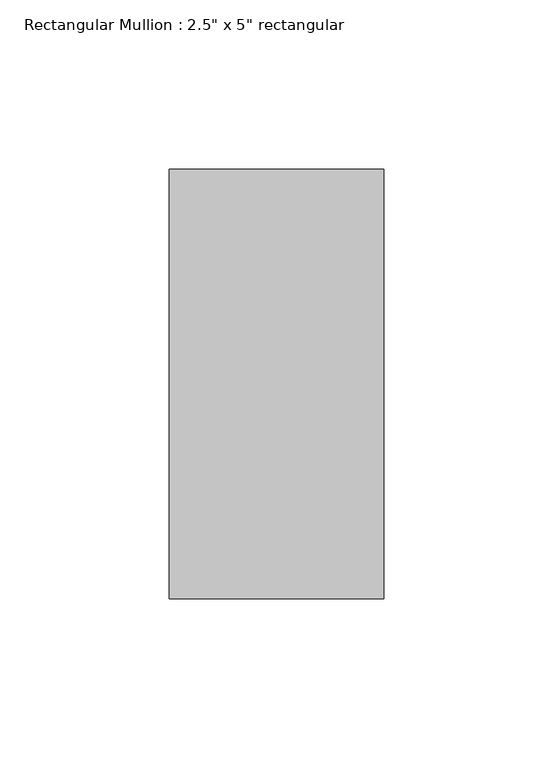
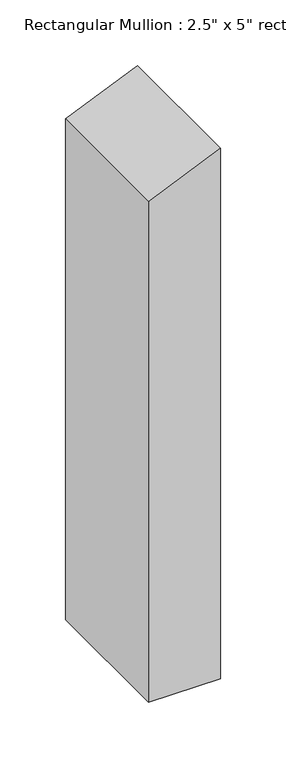
"""IFC4 building model written with IfcOpenShell, lengths in millimetres: member geometry."""

from ifc_helpers import new_model, si_unit, frame, origin, place, context, project, spatial, polyline, outline, extrude, source, transform, mapped, element, save


def member_3f5ee701(model_context):
    return source(origin(), model_context, "Body", "SweptSolid", [
        extrude(outline(polyline([(0.0, 0.0), (-27.6105858, -63.5), (-494.323108, -63.5), (-494.323108, 0.0), (0.0, 0.0)])), frame((0.0, -63.5, 0.0), z_axis=(0.0, 1.0, 0.0), x_axis=(0.0, 0.0, 1.0)), (0.0, 0.0, 1.0), 127.0),
    ])


if __name__ == "__main__":
    model = new_model("IFC4")
    model_context = context("Model", 3, world=origin())
    ifc_project = project(units=[si_unit("LENGTHUNIT", "METRE", prefix="MILLI")], contexts=[model_context])
    site = spatial("IfcSite", under=ifc_project)
    building = spatial("IfcBuilding", under=site)
    placement = place(None, origin())
    member_shape = member_3f5ee701(model_context)
    element("IfcMember", 1, ObjectType="Rectangular Mullion : 2.5\" x 5\" rectangular", at=placement, inside=building, context=model_context, shape_type="MappedRepresentation", body=[
        mapped(member_shape, transform((0.0, 0.0, 0.0), x_axis=(1.0, 0.0, 0.0), y_axis=(0.0, 1.0, 0.0), z_axis=(0.0, 0.0, 1.0))),
    ])
    save(model, "model.ifc")

# Revit data of these elements
# Type "Rectangular Mullion : 2.5\" x 5\" rectangular"
#   built-in parameter 1007304 = 0.416667 (stored number, unit not read)
#   built-in parameter 1007301 = 0.104167 (stored number, unit not read)
#   built-in parameter 1007300 = 0.104167 (stored number, unit not read)
# Element 1 (IfcMember, "Rectangular Mullion : 2.5\" x 5\" rectangular")
#   Materials on its faces: "door colour"
# Materials
#   "door colour": class "Generic", colour RGB 120 120 120, transparency 0, Cost = 0
